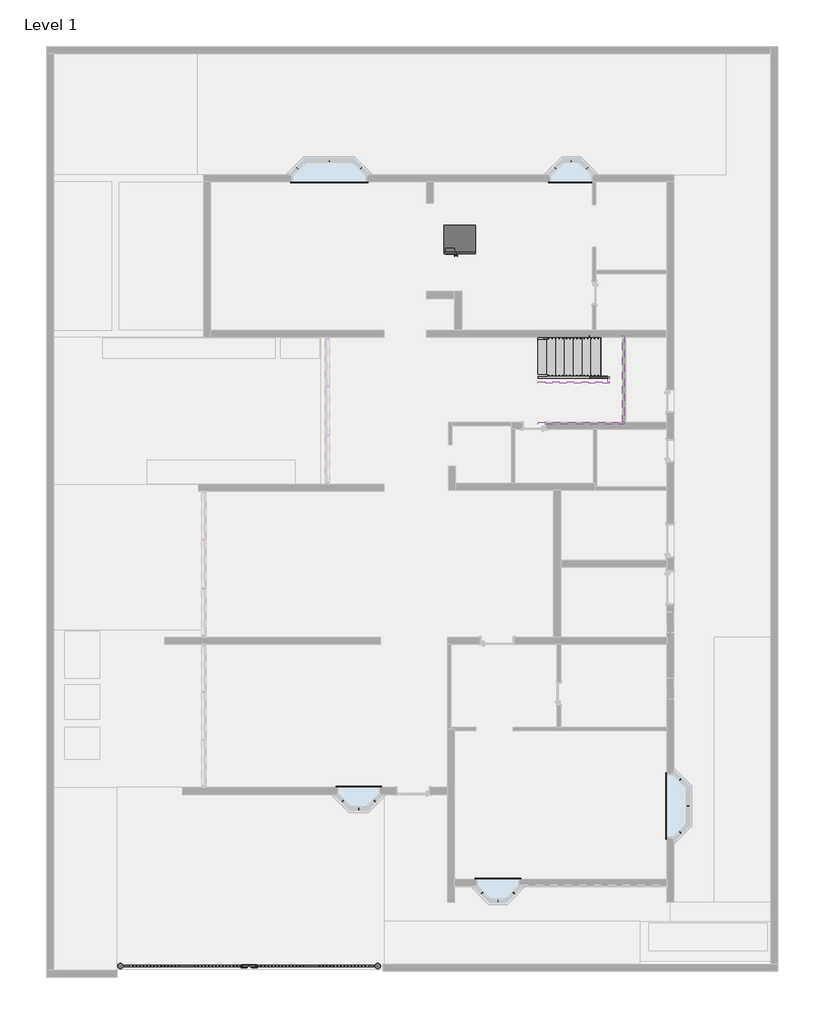
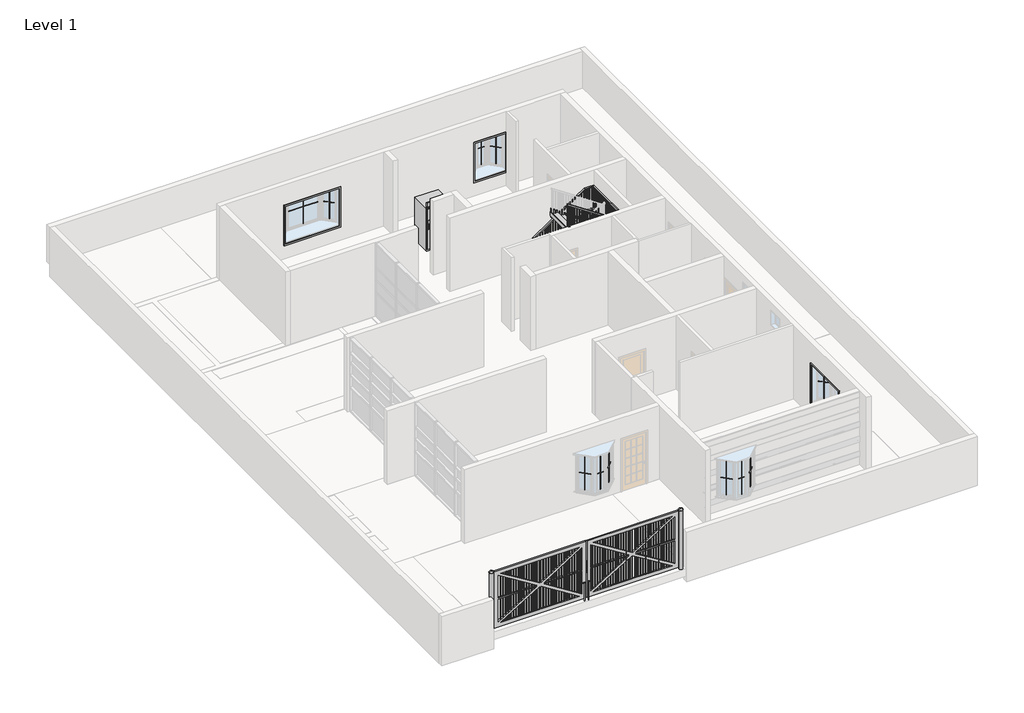
# One storey, part 5 of 5: 22 proxies, 6 members, 1 railing, 1 stair flight.
"""IFC4 building model written with IfcOpenShell, lengths in millimetres."""

from ifc_helpers import new_model, si_unit, frame, origin, place, context, project, spatial, polyline, outline, extrude, faceted_brep, transform, mapped, element, save
from components import proxy_94deb4ca, double_metal_gate_10830_double_metal_gate_10830_8bfe90f4, muntin_pattern_2x2_muntin_pattern_2x2_511ed329, muntin_pattern_2x2_muntin_pattern_2x2_63bd3b25, muntin_pattern_2x2_muntin_pattern_2x2_79566686, muntin_pattern_2x2_muntin_pattern_2x2_fa156a83, trim_window_interior_flat_picture_frame_e25f2530, trim_window_interior_flat_picture_frame_1060724f, trim_window_interior_flat_picture_frame_bf12a1e4, stair_flight_b7e44e04

model = new_model("IFC4")

# Units and contexts
model_context = context("Model", 3, world=origin())
ifc_project = project(units=[si_unit("LENGTHUNIT", "METRE", prefix="MILLI")], contexts=[model_context])

# Site, building, storey
site = spatial("IfcSite", under=ifc_project)
building = spatial("IfcBuilding", under=site)
storey = spatial("IfcBuildingStorey", under=building, Name="Level 1", Elevation=0.0)

# Proxies
placement = place(None, origin())
proxy_shape = proxy_94deb4ca(model_context)
element("IfcBuildingElementProxy", 1, Name="36\" x 70\"", ObjectType="36\" x 70\"", at=placement, inside=storey, context=model_context, shape_type="MappedRepresentation", body=[
    mapped(proxy_shape, transform((-43399.9341626, 8623.3217021, 0.0), x_axis=(1.0, 0.0, 0.0), y_axis=(0.0, 1.0, 0.0), z_axis=(0.0, 0.0, 1.0))),
])
double_metal_gate_10830_double_metal_gate_10830_shape = double_metal_gate_10830_double_metal_gate_10830_8bfe90f4(model_context)
element("IfcBuildingElementProxy", 2, Name="DOUBLE_METAL_GATE_10830 : DOUBLE_METAL_GATE_10830", ObjectType="DOUBLE_METAL_GATE_10830 : DOUBLE_METAL_GATE_10830", at=placement, inside=storey, context=model_context, shape_type="MappedRepresentation", body=[
    mapped(double_metal_gate_10830_double_metal_gate_10830_shape, transform((-48692.8486938, -12363.2913973, 0.0), x_axis=(1.0, 0.0, 0.0), y_axis=(0.0, 1.0, 0.0), z_axis=(0.0, 0.0, 1.0))),
])
muntin_pattern_2x2_muntin_pattern_2x2_shape = muntin_pattern_2x2_muntin_pattern_2x2_511ed329(model_context)
element("IfcBuildingElementProxy", 3, Name="Muntin Pattern_2x2 : Muntin Pattern_2x2", ObjectType="Muntin Pattern_2x2 : Muntin Pattern_2x2", at=placement, inside=storey, context=model_context, shape_type="MappedRepresentation", body=[
    mapped(muntin_pattern_2x2_muntin_pattern_2x2_shape, transform((-47152.5380314, 10861.8336027, 730.25), x_axis=(1.0, 0.0, 0.0), y_axis=(0.0, 1.0, 0.0), z_axis=(0.0, 0.0, 1.0))),
])
muntin_pattern_2x2_muntin_pattern_2x2_2_shape = muntin_pattern_2x2_muntin_pattern_2x2_63bd3b25(model_context)
element("IfcBuildingElementProxy", 4, Name="Muntin Pattern_2x2 : Muntin Pattern_2x2", ObjectType="Muntin Pattern_2x2 : Muntin Pattern_2x2", at=placement, inside=storey, context=model_context, shape_type="MappedRepresentation", body=[
    mapped(muntin_pattern_2x2_muntin_pattern_2x2_2_shape, transform((-48067.2297602, 10633.9378984, 730.25), x_axis=(0.7071067811865505, 0.7071067811865448, 0.0), y_axis=(-0.7071067811865448, 0.7071067811865505, 0.0), z_axis=(0.0, 0.0, 1.0))),
])
element("IfcBuildingElementProxy", 5, Name="Muntin Pattern_2x2 : Muntin Pattern_2x2", ObjectType="Muntin Pattern_2x2 : Muntin Pattern_2x2", at=placement, inside=storey, context=model_context, shape_type="MappedRepresentation", body=[
    mapped(muntin_pattern_2x2_muntin_pattern_2x2_2_shape, transform((-46237.8463026, 10633.9378984, 730.25), x_axis=(0.707106781186546, -0.7071067811865491, 0.0), y_axis=(0.7071067811865491, 0.707106781186546, 0.0), z_axis=(0.0, 0.0, 1.0))),
])
element("IfcBuildingElementProxy", 6, Name="Muntin Pattern_2x2 : Muntin Pattern_2x2", ObjectType="Muntin Pattern_2x2 : Muntin Pattern_2x2", at=placement, inside=storey, context=model_context, shape_type="MappedRepresentation", body=[
    mapped(muntin_pattern_2x2_muntin_pattern_2x2_2_shape, transform((-40650.4297602, 10633.9378984, 730.25), x_axis=(0.7071067811865505, 0.7071067811865448, 0.0), y_axis=(-0.7071067811865448, 0.7071067811865505, 0.0), z_axis=(0.0, 0.0, 1.0))),
])
element("IfcBuildingElementProxy", 7, Name="Muntin Pattern_2x2 : Muntin Pattern_2x2", ObjectType="Muntin Pattern_2x2 : Muntin Pattern_2x2", at=placement, inside=storey, context=model_context, shape_type="MappedRepresentation", body=[
    mapped(muntin_pattern_2x2_muntin_pattern_2x2_2_shape, transform((-39735.4463026, 10633.9378984, 730.25), x_axis=(0.707106781186546, -0.7071067811865491, 0.0), y_axis=(0.7071067811865491, 0.707106781186546, 0.0), z_axis=(0.0, 0.0, 1.0))),
])
element("IfcBuildingElementProxy", 8, Name="Muntin Pattern_2x2 : Muntin Pattern_2x2", ObjectType="Muntin Pattern_2x2 : Muntin Pattern_2x2", at=placement, inside=storey, context=model_context, shape_type="MappedRepresentation", body=[
    mapped(muntin_pattern_2x2_muntin_pattern_2x2_2_shape, transform((-41843.6463026, -10189.1206929, 730.25), x_axis=(-0.7071067811865505, -0.7071067811865448, 0.0), y_axis=(0.7071067811865448, -0.7071067811865505, 0.0), z_axis=(0.0, 0.0, 1.0))),
])
element("IfcBuildingElementProxy", 9, Name="Muntin Pattern_2x2 : Muntin Pattern_2x2", ObjectType="Muntin Pattern_2x2 : Muntin Pattern_2x2", at=placement, inside=storey, context=model_context, shape_type="MappedRepresentation", body=[
    mapped(muntin_pattern_2x2_muntin_pattern_2x2_2_shape, transform((-42758.6297602, -10189.1206929, 730.25), x_axis=(-0.707106781186546, 0.7071067811865491, 0.0), y_axis=(-0.7071067811865491, -0.707106781186546, 0.0), z_axis=(0.0, 0.0, 1.0))),
])
element("IfcBuildingElementProxy", 10, Name="Muntin Pattern_2x2 : Muntin Pattern_2x2", ObjectType="Muntin Pattern_2x2 : Muntin Pattern_2x2", at=placement, inside=storey, context=model_context, shape_type="MappedRepresentation", body=[
    mapped(muntin_pattern_2x2_muntin_pattern_2x2_2_shape, transform((-37058.5087357, -6927.3996684, 730.25), x_axis=(0.7071067811865458, -0.7071067811865495, 0.0), y_axis=(0.7071067811865495, 0.7071067811865458, 0.0), z_axis=(0.0, 0.0, 1.0))),
])
element("IfcBuildingElementProxy", 11, Name="Muntin Pattern_2x2 : Muntin Pattern_2x2", ObjectType="Muntin Pattern_2x2 : Muntin Pattern_2x2", at=placement, inside=storey, context=model_context, shape_type="MappedRepresentation", body=[
    mapped(muntin_pattern_2x2_muntin_pattern_2x2_2_shape, transform((-37058.5087357, -8451.9831261, 730.25), x_axis=(-0.7071067811865481, -0.707106781186547, 0.0), y_axis=(0.707106781186547, -0.7071067811865481, 0.0), z_axis=(0.0, 0.0, 1.0))),
])
element("IfcBuildingElementProxy", 12, Name="Muntin Pattern_2x2 : Muntin Pattern_2x2", ObjectType="Muntin Pattern_2x2 : Muntin Pattern_2x2", at=placement, inside=storey, context=model_context, shape_type="MappedRepresentation", body=[
    mapped(muntin_pattern_2x2_muntin_pattern_2x2_2_shape, transform((-45844.1463026, -7547.5206929, 730.25), x_axis=(-0.7071067811865506, -0.7071067811865447, 0.0), y_axis=(0.7071067811865447, -0.7071067811865506, 0.0), z_axis=(0.0, 0.0, 1.0))),
])
element("IfcBuildingElementProxy", 13, Name="Muntin Pattern_2x2 : Muntin Pattern_2x2", ObjectType="Muntin Pattern_2x2 : Muntin Pattern_2x2", at=placement, inside=storey, context=model_context, shape_type="MappedRepresentation", body=[
    mapped(muntin_pattern_2x2_muntin_pattern_2x2_2_shape, transform((-46759.1297602, -7547.5206929, 730.25), x_axis=(-0.7071067811865459, 0.7071067811865492, 0.0), y_axis=(-0.7071067811865492, -0.7071067811865459, 0.0), z_axis=(0.0, 0.0, 1.0))),
])
muntin_pattern_2x2_muntin_pattern_2x2_3_shape = muntin_pattern_2x2_muntin_pattern_2x2_79566686(model_context)
element("IfcBuildingElementProxy", 14, Name="Muntin Pattern_2x2 : Muntin Pattern_2x2", ObjectType="Muntin Pattern_2x2 : Muntin Pattern_2x2", at=placement, inside=storey, context=model_context, shape_type="MappedRepresentation", body=[
    mapped(muntin_pattern_2x2_muntin_pattern_2x2_3_shape, transform((-40192.9380314, 10861.8336027, 730.25), x_axis=(1.0, 0.0, 0.0), y_axis=(0.0, 1.0, 0.0), z_axis=(0.0, 0.0, 1.0))),
])
element("IfcBuildingElementProxy", 15, Name="Muntin Pattern_2x2 : Muntin Pattern_2x2", ObjectType="Muntin Pattern_2x2 : Muntin Pattern_2x2", at=placement, inside=storey, context=model_context, shape_type="MappedRepresentation", body=[
    mapped(muntin_pattern_2x2_muntin_pattern_2x2_3_shape, transform((-42301.1380314, -10417.0163973, 730.25), x_axis=(-1.0, 0.0, 0.0), y_axis=(0.0, -1.0, 0.0), z_axis=(0.0, 0.0, 1.0))),
])
element("IfcBuildingElementProxy", 16, Name="Muntin Pattern_2x2 : Muntin Pattern_2x2", ObjectType="Muntin Pattern_2x2 : Muntin Pattern_2x2", at=placement, inside=storey, context=model_context, shape_type="MappedRepresentation", body=[
    mapped(muntin_pattern_2x2_muntin_pattern_2x2_3_shape, transform((-46301.6380314, -7775.4163973, 730.25), x_axis=(-1.0, 0.0, 0.0), y_axis=(0.0, -1.0, 0.0), z_axis=(0.0, 0.0, 1.0))),
])
muntin_pattern_2x2_muntin_pattern_2x2_4_shape = muntin_pattern_2x2_muntin_pattern_2x2_fa156a83(model_context)
element("IfcBuildingElementProxy", 17, Name="Muntin Pattern_2x2 : Muntin Pattern_2x2", ObjectType="Muntin Pattern_2x2 : Muntin Pattern_2x2", at=placement, inside=storey, context=model_context, shape_type="MappedRepresentation", body=[
    mapped(muntin_pattern_2x2_muntin_pattern_2x2_4_shape, transform((-36830.6130314, -7689.6913973, 730.25), x_axis=(0.0, -1.0, 0.0), y_axis=(1.0, 0.0, 0.0), z_axis=(0.0, 0.0, 1.0))),
])
trim_window_interior_flat_picture_frame_shape = trim_window_interior_flat_picture_frame_e25f2530(model_context)
element("IfcBuildingElementProxy", 18, Name="Trim-Window-Interior-Flat : Picture Frame", ObjectType="Trim-Window-Interior-Flat : Picture Frame", at=placement, inside=storey, context=model_context, shape_type="MappedRepresentation", body=[
    mapped(trim_window_interior_flat_picture_frame_shape, transform((-47152.5380314, 10242.7086027, 2184.4), x_axis=(1.0, 0.0, 0.0), y_axis=(0.0, 0.0, 1.0), z_axis=(0.0, -1.0, 0.0))),
])
trim_window_interior_flat_picture_frame_2_shape = trim_window_interior_flat_picture_frame_1060724f(model_context)
element("IfcBuildingElementProxy", 19, Name="Trim-Window-Interior-Flat : Picture Frame", ObjectType="Trim-Window-Interior-Flat : Picture Frame", at=placement, inside=storey, context=model_context, shape_type="MappedRepresentation", body=[
    mapped(trim_window_interior_flat_picture_frame_2_shape, transform((-40192.9380314, 10242.7086027, 2184.4), x_axis=(1.0, 0.0, 0.0), y_axis=(0.0, 0.0, 1.0), z_axis=(0.0, -1.0, 0.0))),
])
element("IfcBuildingElementProxy", 20, Name="Trim-Window-Interior-Flat : Picture Frame", ObjectType="Trim-Window-Interior-Flat : Picture Frame", at=placement, inside=storey, context=model_context, shape_type="MappedRepresentation", body=[
    mapped(trim_window_interior_flat_picture_frame_2_shape, transform((-42301.1380314, -9797.8913973, 2184.4), x_axis=(-1.0, 0.0, 0.0), y_axis=(0.0, 0.0, 1.0), z_axis=(0.0, 1.0, 0.0))),
])
element("IfcBuildingElementProxy", 21, Name="Trim-Window-Interior-Flat : Picture Frame", ObjectType="Trim-Window-Interior-Flat : Picture Frame", at=placement, inside=storey, context=model_context, shape_type="MappedRepresentation", body=[
    mapped(trim_window_interior_flat_picture_frame_2_shape, transform((-46301.6380314, -7156.2913973, 2184.4), x_axis=(-1.0, 0.0, 0.0), y_axis=(0.0, 0.0, 1.0), z_axis=(0.0, 1.0, 0.0))),
])
trim_window_interior_flat_picture_frame_3_shape = trim_window_interior_flat_picture_frame_bf12a1e4(model_context)
element("IfcBuildingElementProxy", 22, Name="Trim-Window-Interior-Flat : Picture Frame", ObjectType="Trim-Window-Interior-Flat : Picture Frame", at=placement, inside=storey, context=model_context, shape_type="MappedRepresentation", body=[
    mapped(trim_window_interior_flat_picture_frame_3_shape, transform((-37449.7380314, -7689.6913973, 2184.4), x_axis=(0.0, -1.0, 0.0), y_axis=(0.0, 0.0, 1.0), z_axis=(-1.0, 0.0, 0.0))),
])

# Members
element("IfcMember", 23, ObjectType="Stringer - 2\" Width", at=placement, inside=storey, context=model_context, shape_type="SweptSolid", body=[
    extrude(outline(polyline([(218.0398409, -41148.2472477), (0.0, -41148.2472477), (0.0, -40925.8209948), (1470.7219756, -38719.7380314), (1600.2, -38719.7380314), (1600.2, -39075.0070091), (218.0398409, -41148.2472477)])), frame((0.0, 5772.3086027, 0.0), z_axis=(0.0, 1.0, 0.0), x_axis=(0.0, 0.0, 1.0)), (0.0, 0.0, 1.0), 50.8),
])
element("IfcMember", 24, ObjectType="Stringer - 2\" Width", at=placement, inside=storey, context=model_context, shape_type="SweptSolid", body=[
    extrude(outline(polyline([(-38719.7380314, 5823.1086027), (-38668.9380314, 5823.1086027), (-38668.9380314, 3333.9086027), (-38719.7380314, 3333.9086027), (-38719.7380314, 5823.1086027)])), frame((0.0, 0.0, 1295.4), z_axis=(0.0, 0.0, 1.0), x_axis=(1.0, 0.0, 0.0)), (0.0, 0.0, 1.0), 304.8),
])
element("IfcMember", 25, ObjectType="Stringer - 2\" Width", at=placement, inside=storey, context=model_context, shape_type="SweptSolid", body=[
    extrude(outline(polyline([(1295.4, -38668.9380314), (1443.8336967, -38668.9380314), (3096.7065076, -41148.2472477), (2730.382498, -41148.2472477), (1295.4, -38995.7735007), (1295.4, -38668.9380314)])), frame((0.0, 3283.1086027, 0.0), z_axis=(0.0, 1.0, 0.0), x_axis=(0.0, 0.0, 1.0)), (0.0, 0.0, 1.0), 50.8),
])
element("IfcMember", 26, ObjectType="Stringer - 2\" Width", at=placement, inside=storey, context=model_context, shape_type="SweptSolid", body=[
    extrude(outline(polyline([(218.0398409, -41148.2472477), (0.0, -41148.2472477), (0.0, -40925.8209948), (1189.4491647, -39141.6472477), (1555.7731743, -39141.6472477), (218.0398409, -41148.2472477)])), frame((0.0, 4603.9086027, 0.0), z_axis=(0.0, 1.0, 0.0), x_axis=(0.0, 0.0, 1.0)), (0.0, 0.0, 1.0), 50.8),
])
element("IfcMember", 27, ObjectType="Stringer - 2\" Width", at=placement, inside=storey, context=model_context, shape_type="SweptSolid", body=[
    extrude(outline(polyline([(-39141.6472477, 4654.7086027), (-39090.8472477, 4654.7086027), (-39090.8472477, 4502.3086027), (-39141.6472477, 4502.3086027), (-39141.6472477, 4654.7086027)])), frame((0.0, 0.0, 1295.4), z_axis=(0.0, 0.0, 1.0), x_axis=(1.0, 0.0, 0.0)), (0.0, 0.0, 1.0), 304.8),
])
element("IfcMember", 28, ObjectType="Stringer - 2\" Width", at=placement, inside=storey, context=model_context, shape_type="SweptSolid", body=[
    extrude(outline(polyline([(1358.782498, -39090.8472477), (1725.1065076, -39090.8472477), (3096.7065076, -41148.2472477), (2730.382498, -41148.2472477), (1358.782498, -39090.8472477)])), frame((0.0, 4451.5086027, 0.0), z_axis=(0.0, 1.0, 0.0), x_axis=(0.0, 0.0, 1.0)), (0.0, 0.0, 1.0), 50.8),
])

# Railing
element("IfcRailing", 29, ObjectType="Handrail - Rectangular", at=placement, inside=storey, context=model_context, shape_type="SolidModel", body=[
    faceted_brep([(-41148.2472477, 5772.3086027, 1083.7333333), (-41148.2472477, 5772.3086027, 1022.6793317), (-41148.2472477, 5721.5086027, 1022.6793317), (-41148.2472477, 5721.5086027, 1083.7333333), (-39116.2472477, 5772.3086027, 2438.4), (-39100.8662454, 5772.3086027, 2387.6), (-39100.8662454, 5721.5086027, 2387.6), (-39116.2472477, 5721.5086027, 2438.4), (-38719.7380314, 5772.3086027, 2438.4), (-38719.7380314, 5772.3086027, 2387.6), (-38770.5380314, 5721.5086027, 2387.6), (-38770.5380314, 5721.5086027, 2438.4), (-38719.7380314, 3333.9086027, 2438.4), (-38719.7380314, 3333.9086027, 2387.6), (-38770.5380314, 3384.7086027, 2387.6), (-38770.5380314, 3384.7086027, 2438.4), (-38862.2472477, 3333.9086027, 2438.4), (-38877.6282501, 3333.9086027, 2387.6), (-38877.6282501, 3384.7086027, 2387.6), (-38862.2472477, 3384.7086027, 2438.4), (-41148.2472477, 3333.9086027, 3962.4), (-41148.2472477, 3384.7086027, 3962.4), (-41148.2472477, 3384.7086027, 3901.3459984), (-41148.2472477, 3333.9086027, 3901.3459984)], [[[0, 1, 2, 3]], [[1, 0, 4, 5]], [[2, 1, 5, 6]], [[3, 2, 6, 7]], [[0, 3, 7, 4]], [[5, 4, 8, 9]], [[6, 5, 9, 10]], [[7, 6, 10, 11]], [[4, 7, 11, 8]], [[9, 8, 12, 13]], [[10, 9, 13, 14]], [[11, 10, 14, 15]], [[8, 11, 15, 12]], [[13, 12, 16, 17]], [[14, 13, 17, 18]], [[15, 14, 18, 19]], [[12, 15, 19, 16]], [[20, 21, 22, 23]], [[17, 16, 20, 23]], [[18, 17, 23, 22]], [[19, 18, 22, 21]], [[16, 19, 21, 20]]]),
    extrude(outline(polyline([(3863.4898542, -41091.4630314), (2878.6666667, -41091.4630314), (2878.6666667, -41072.4130314), (3850.7898542, -41072.4130314), (3863.4898542, -41091.4630314)])), frame((0.0, 3349.7836027, 0.0), z_axis=(0.0, 1.0, 0.0), x_axis=(0.0, 0.0, 1.0)), (0.0, 0.0, 1.0), 19.05),
    extrude(outline(polyline([(3795.7565208, -40989.8630314), (2878.6666667, -40989.8630314), (2878.6666667, -40970.8130314), (3783.0565208, -40970.8130314), (3795.7565208, -40989.8630314)])), frame((0.0, 3349.7836027, 0.0), z_axis=(0.0, 1.0, 0.0), x_axis=(0.0, 0.0, 1.0)), (0.0, 0.0, 1.0), 19.05),
    extrude(outline(polyline([(3728.0231875, -40888.2630314), (2709.3333333, -40888.2630314), (2709.3333333, -40869.2130314), (3715.3231875, -40869.2130314), (3728.0231875, -40888.2630314)])), frame((0.0, 3349.7836027, 0.0), z_axis=(0.0, 1.0, 0.0), x_axis=(0.0, 0.0, 1.0)), (0.0, 0.0, 1.0), 19.05),
    extrude(outline(polyline([(3660.2898542, -40786.6630314), (2709.3333333, -40786.6630314), (2709.3333333, -40767.6130314), (3647.5898542, -40767.6130314), (3660.2898542, -40786.6630314)])), frame((0.0, 3349.7836027, 0.0), z_axis=(0.0, 1.0, 0.0), x_axis=(0.0, 0.0, 1.0)), (0.0, 0.0, 1.0), 19.05),
    extrude(outline(polyline([(3592.5565208, -40685.0630314), (2709.3333333, -40685.0630314), (2709.3333333, -40666.0130314), (3579.8565208, -40666.0130314), (3592.5565208, -40685.0630314)])), frame((0.0, 3349.7836027, 0.0), z_axis=(0.0, 1.0, 0.0), x_axis=(0.0, 0.0, 1.0)), (0.0, 0.0, 1.0), 19.05),
    extrude(outline(polyline([(3524.8231875, -40583.4630314), (2540.0, -40583.4630314), (2540.0, -40564.4130314), (3512.1231875, -40564.4130314), (3524.8231875, -40583.4630314)])), frame((0.0, 3349.7836027, 0.0), z_axis=(0.0, 1.0, 0.0), x_axis=(0.0, 0.0, 1.0)), (0.0, 0.0, 1.0), 19.05),
    extrude(outline(polyline([(3457.0898542, -40481.8630314), (2540.0, -40481.8630314), (2540.0, -40462.8130314), (3444.3898542, -40462.8130314), (3457.0898542, -40481.8630314)])), frame((0.0, 3349.7836027, 0.0), z_axis=(0.0, 1.0, 0.0), x_axis=(0.0, 0.0, 1.0)), (0.0, 0.0, 1.0), 19.05),
    extrude(outline(polyline([(3389.3565208, -40380.2630314), (2370.6666667, -40380.2630314), (2370.6666667, -40361.2130314), (3376.6565208, -40361.2130314), (3389.3565208, -40380.2630314)])), frame((0.0, 3349.7836027, 0.0), z_axis=(0.0, 1.0, 0.0), x_axis=(0.0, 0.0, 1.0)), (0.0, 0.0, 1.0), 19.05),
    extrude(outline(polyline([(3321.6231875, -40278.6630314), (2370.6666667, -40278.6630314), (2370.6666667, -40259.6130314), (3308.9231875, -40259.6130314), (3321.6231875, -40278.6630314)])), frame((0.0, 3349.7836027, 0.0), z_axis=(0.0, 1.0, 0.0), x_axis=(0.0, 0.0, 1.0)), (0.0, 0.0, 1.0), 19.05),
    extrude(outline(polyline([(3253.8898542, -40177.0630314), (2370.6666667, -40177.0630314), (2370.6666667, -40158.0130314), (3241.1898542, -40158.0130314), (3253.8898542, -40177.0630314)])), frame((0.0, 3349.7836027, 0.0), z_axis=(0.0, 1.0, 0.0), x_axis=(0.0, 0.0, 1.0)), (0.0, 0.0, 1.0), 19.05),
    extrude(outline(polyline([(3186.1565208, -40075.4630314), (2201.3333333, -40075.4630314), (2201.3333333, -40056.4130314), (3173.4565208, -40056.4130314), (3186.1565208, -40075.4630314)])), frame((0.0, 3349.7836027, 0.0), z_axis=(0.0, 1.0, 0.0), x_axis=(0.0, 0.0, 1.0)), (0.0, 0.0, 1.0), 19.05),
    extrude(outline(polyline([(3118.4231875, -39973.8630314), (2201.3333333, -39973.8630314), (2201.3333333, -39954.8130314), (3105.7231875, -39954.8130314), (3118.4231875, -39973.8630314)])), frame((0.0, 3349.7836027, 0.0), z_axis=(0.0, 1.0, 0.0), x_axis=(0.0, 0.0, 1.0)), (0.0, 0.0, 1.0), 19.05),
    extrude(outline(polyline([(3050.6898542, -39872.2630314), (2032.0, -39872.2630314), (2032.0, -39853.2130314), (3037.9898542, -39853.2130314), (3050.6898542, -39872.2630314)])), frame((0.0, 3349.7836027, 0.0), z_axis=(0.0, 1.0, 0.0), x_axis=(0.0, 0.0, 1.0)), (0.0, 0.0, 1.0), 19.05),
    extrude(outline(polyline([(2982.9565208, -39770.6630314), (2032.0, -39770.6630314), (2032.0, -39751.6130314), (2970.2565208, -39751.6130314), (2982.9565208, -39770.6630314)])), frame((0.0, 3349.7836027, 0.0), z_axis=(0.0, 1.0, 0.0), x_axis=(0.0, 0.0, 1.0)), (0.0, 0.0, 1.0), 19.05),
    extrude(outline(polyline([(2915.2231875, -39669.0630314), (2032.0, -39669.0630314), (2032.0, -39650.0130314), (2902.5231875, -39650.0130314), (2915.2231875, -39669.0630314)])), frame((0.0, 3349.7836027, 0.0), z_axis=(0.0, 1.0, 0.0), x_axis=(0.0, 0.0, 1.0)), (0.0, 0.0, 1.0), 19.05),
    extrude(outline(polyline([(2847.4898542, -39567.4630314), (1862.6666667, -39567.4630314), (1862.6666667, -39548.4130314), (2834.7898542, -39548.4130314), (2847.4898542, -39567.4630314)])), frame((0.0, 3349.7836027, 0.0), z_axis=(0.0, 1.0, 0.0), x_axis=(0.0, 0.0, 1.0)), (0.0, 0.0, 1.0), 19.05),
    extrude(outline(polyline([(2779.7565208, -39465.8630314), (1862.6666667, -39465.8630314), (1862.6666667, -39446.8130314), (2767.0565208, -39446.8130314), (2779.7565208, -39465.8630314)])), frame((0.0, 3349.7836027, 0.0), z_axis=(0.0, 1.0, 0.0), x_axis=(0.0, 0.0, 1.0)), (0.0, 0.0, 1.0), 19.05),
    extrude(outline(polyline([(2712.0231875, -39364.2630314), (1693.3333333, -39364.2630314), (1693.3333333, -39345.2130314), (2699.3231875, -39345.2130314), (2712.0231875, -39364.2630314)])), frame((0.0, 3349.7836027, 0.0), z_axis=(0.0, 1.0, 0.0), x_axis=(0.0, 0.0, 1.0)), (0.0, 0.0, 1.0), 19.05),
    extrude(outline(polyline([(2644.2898542, -39262.6630314), (1693.3333333, -39262.6630314), (1693.3333333, -39243.6130314), (2631.5898542, -39243.6130314), (2644.2898542, -39262.6630314)])), frame((0.0, 3349.7836027, 0.0), z_axis=(0.0, 1.0, 0.0), x_axis=(0.0, 0.0, 1.0)), (0.0, 0.0, 1.0), 19.05),
    extrude(outline(polyline([(2576.5565208, -39161.0630314), (1693.3333333, -39161.0630314), (1693.3333333, -39142.0130314), (2563.8565208, -39142.0130314), (2576.5565208, -39161.0630314)])), frame((0.0, 3349.7836027, 0.0), z_axis=(0.0, 1.0, 0.0), x_axis=(0.0, 0.0, 1.0)), (0.0, 0.0, 1.0), 19.05),
    extrude(outline(polyline([(2508.8231875, -39059.4630314), (1524.0, -39059.4630314), (1524.0, -39040.4130314), (2496.1231875, -39040.4130314), (2508.8231875, -39059.4630314)])), frame((0.0, 3349.7836027, 0.0), z_axis=(0.0, 1.0, 0.0), x_axis=(0.0, 0.0, 1.0)), (0.0, 0.0, 1.0), 19.05),
    extrude(outline(polyline([(2441.0898542, -38957.8630314), (1524.0, -38957.8630314), (1524.0, -38938.8130314), (2428.3898542, -38938.8130314), (2441.0898542, -38957.8630314)])), frame((0.0, 3349.7836027, 0.0), z_axis=(0.0, 1.0, 0.0), x_axis=(0.0, 0.0, 1.0)), (0.0, 0.0, 1.0), 19.05),
    extrude(outline(polyline([(-38837.2130314, 3349.7836027), (-38856.2630314, 3349.7836027), (-38856.2630314, 3368.8336027), (-38837.2130314, 3368.8336027), (-38837.2130314, 3349.7836027)])), frame((0.0, 0.0, 1524.0), z_axis=(0.0, 0.0, 1.0), x_axis=(1.0, 0.0, 0.0)), (0.0, 0.0, 1.0), 863.6),
    extrude(outline(polyline([(-38735.6130314, 3419.6336027), (-38735.6130314, 3400.5836027), (-38754.6630314, 3400.5836027), (-38754.6630314, 3419.6336027), (-38735.6130314, 3419.6336027)])), frame((0.0, 0.0, 1524.0), z_axis=(0.0, 0.0, 1.0), x_axis=(1.0, 0.0, 0.0)), (0.0, 0.0, 1.0), 863.6),
    extrude(outline(polyline([(-38735.6130314, 3521.2336027), (-38735.6130314, 3502.1836027), (-38754.6630314, 3502.1836027), (-38754.6630314, 3521.2336027), (-38735.6130314, 3521.2336027)])), frame((0.0, 0.0, 1524.0), z_axis=(0.0, 0.0, 1.0), x_axis=(1.0, 0.0, 0.0)), (0.0, 0.0, 1.0), 863.6),
    extrude(outline(polyline([(-38735.6130314, 3622.8336027), (-38735.6130314, 3603.7836027), (-38754.6630314, 3603.7836027), (-38754.6630314, 3622.8336027), (-38735.6130314, 3622.8336027)])), frame((0.0, 0.0, 1524.0), z_axis=(0.0, 0.0, 1.0), x_axis=(1.0, 0.0, 0.0)), (0.0, 0.0, 1.0), 863.6),
    extrude(outline(polyline([(-38735.6130314, 3724.4336027), (-38735.6130314, 3705.3836027), (-38754.6630314, 3705.3836027), (-38754.6630314, 3724.4336027), (-38735.6130314, 3724.4336027)])), frame((0.0, 0.0, 1524.0), z_axis=(0.0, 0.0, 1.0), x_axis=(1.0, 0.0, 0.0)), (0.0, 0.0, 1.0), 863.6),
    extrude(outline(polyline([(-38735.6130314, 3826.0336027), (-38735.6130314, 3806.9836027), (-38754.6630314, 3806.9836027), (-38754.6630314, 3826.0336027), (-38735.6130314, 3826.0336027)])), frame((0.0, 0.0, 1524.0), z_axis=(0.0, 0.0, 1.0), x_axis=(1.0, 0.0, 0.0)), (0.0, 0.0, 1.0), 863.6),
    extrude(outline(polyline([(-38735.6130314, 3927.6336027), (-38735.6130314, 3908.5836027), (-38754.6630314, 3908.5836027), (-38754.6630314, 3927.6336027), (-38735.6130314, 3927.6336027)])), frame((0.0, 0.0, 1524.0), z_axis=(0.0, 0.0, 1.0), x_axis=(1.0, 0.0, 0.0)), (0.0, 0.0, 1.0), 863.6),
    extrude(outline(polyline([(-38735.6130314, 4029.2336027), (-38735.6130314, 4010.1836027), (-38754.6630314, 4010.1836027), (-38754.6630314, 4029.2336027), (-38735.6130314, 4029.2336027)])), frame((0.0, 0.0, 1524.0), z_axis=(0.0, 0.0, 1.0), x_axis=(1.0, 0.0, 0.0)), (0.0, 0.0, 1.0), 863.6),
    extrude(outline(polyline([(-38735.6130314, 4130.8336027), (-38735.6130314, 4111.7836027), (-38754.6630314, 4111.7836027), (-38754.6630314, 4130.8336027), (-38735.6130314, 4130.8336027)])), frame((0.0, 0.0, 1524.0), z_axis=(0.0, 0.0, 1.0), x_axis=(1.0, 0.0, 0.0)), (0.0, 0.0, 1.0), 863.6),
    extrude(outline(polyline([(-38735.6130314, 4232.4336027), (-38735.6130314, 4213.3836027), (-38754.6630314, 4213.3836027), (-38754.6630314, 4232.4336027), (-38735.6130314, 4232.4336027)])), frame((0.0, 0.0, 1524.0), z_axis=(0.0, 0.0, 1.0), x_axis=(1.0, 0.0, 0.0)), (0.0, 0.0, 1.0), 863.6),
    extrude(outline(polyline([(-38735.6130314, 4334.0336027), (-38735.6130314, 4314.9836027), (-38754.6630314, 4314.9836027), (-38754.6630314, 4334.0336027), (-38735.6130314, 4334.0336027)])), frame((0.0, 0.0, 1524.0), z_axis=(0.0, 0.0, 1.0), x_axis=(1.0, 0.0, 0.0)), (0.0, 0.0, 1.0), 863.6),
    extrude(outline(polyline([(-38735.6130314, 4435.6336027), (-38735.6130314, 4416.5836027), (-38754.6630314, 4416.5836027), (-38754.6630314, 4435.6336027), (-38735.6130314, 4435.6336027)])), frame((0.0, 0.0, 1524.0), z_axis=(0.0, 0.0, 1.0), x_axis=(1.0, 0.0, 0.0)), (0.0, 0.0, 1.0), 863.6),
    extrude(outline(polyline([(-38735.6130314, 4537.2336027), (-38735.6130314, 4518.1836027), (-38754.6630314, 4518.1836027), (-38754.6630314, 4537.2336027), (-38735.6130314, 4537.2336027)])), frame((0.0, 0.0, 1524.0), z_axis=(0.0, 0.0, 1.0), x_axis=(1.0, 0.0, 0.0)), (0.0, 0.0, 1.0), 863.6),
    extrude(outline(polyline([(-38735.6130314, 4638.8336027), (-38735.6130314, 4619.7836027), (-38754.6630314, 4619.7836027), (-38754.6630314, 4638.8336027), (-38735.6130314, 4638.8336027)])), frame((0.0, 0.0, 1524.0), z_axis=(0.0, 0.0, 1.0), x_axis=(1.0, 0.0, 0.0)), (0.0, 0.0, 1.0), 863.6),
    extrude(outline(polyline([(-38735.6130314, 4740.4336027), (-38735.6130314, 4721.3836027), (-38754.6630314, 4721.3836027), (-38754.6630314, 4740.4336027), (-38735.6130314, 4740.4336027)])), frame((0.0, 0.0, 1524.0), z_axis=(0.0, 0.0, 1.0), x_axis=(1.0, 0.0, 0.0)), (0.0, 0.0, 1.0), 863.6),
    extrude(outline(polyline([(-38735.6130314, 4842.0336027), (-38735.6130314, 4822.9836027), (-38754.6630314, 4822.9836027), (-38754.6630314, 4842.0336027), (-38735.6130314, 4842.0336027)])), frame((0.0, 0.0, 1524.0), z_axis=(0.0, 0.0, 1.0), x_axis=(1.0, 0.0, 0.0)), (0.0, 0.0, 1.0), 863.6),
    extrude(outline(polyline([(-38735.6130314, 4943.6336027), (-38735.6130314, 4924.5836027), (-38754.6630314, 4924.5836027), (-38754.6630314, 4943.6336027), (-38735.6130314, 4943.6336027)])), frame((0.0, 0.0, 1524.0), z_axis=(0.0, 0.0, 1.0), x_axis=(1.0, 0.0, 0.0)), (0.0, 0.0, 1.0), 863.6),
    extrude(outline(polyline([(-38735.6130314, 5045.2336027), (-38735.6130314, 5026.1836027), (-38754.6630314, 5026.1836027), (-38754.6630314, 5045.2336027), (-38735.6130314, 5045.2336027)])), frame((0.0, 0.0, 1524.0), z_axis=(0.0, 0.0, 1.0), x_axis=(1.0, 0.0, 0.0)), (0.0, 0.0, 1.0), 863.6),
    extrude(outline(polyline([(-38735.6130314, 5146.8336027), (-38735.6130314, 5127.7836027), (-38754.6630314, 5127.7836027), (-38754.6630314, 5146.8336027), (-38735.6130314, 5146.8336027)])), frame((0.0, 0.0, 1524.0), z_axis=(0.0, 0.0, 1.0), x_axis=(1.0, 0.0, 0.0)), (0.0, 0.0, 1.0), 863.6),
    extrude(outline(polyline([(-38735.6130314, 5248.4336027), (-38735.6130314, 5229.3836027), (-38754.6630314, 5229.3836027), (-38754.6630314, 5248.4336027), (-38735.6130314, 5248.4336027)])), frame((0.0, 0.0, 1524.0), z_axis=(0.0, 0.0, 1.0), x_axis=(1.0, 0.0, 0.0)), (0.0, 0.0, 1.0), 863.6),
    extrude(outline(polyline([(-38735.6130314, 5350.0336027), (-38735.6130314, 5330.9836027), (-38754.6630314, 5330.9836027), (-38754.6630314, 5350.0336027), (-38735.6130314, 5350.0336027)])), frame((0.0, 0.0, 1524.0), z_axis=(0.0, 0.0, 1.0), x_axis=(1.0, 0.0, 0.0)), (0.0, 0.0, 1.0), 863.6),
    extrude(outline(polyline([(-38735.6130314, 5451.6336027), (-38735.6130314, 5432.5836027), (-38754.6630314, 5432.5836027), (-38754.6630314, 5451.6336027), (-38735.6130314, 5451.6336027)])), frame((0.0, 0.0, 1524.0), z_axis=(0.0, 0.0, 1.0), x_axis=(1.0, 0.0, 0.0)), (0.0, 0.0, 1.0), 863.6),
    extrude(outline(polyline([(-38735.6130314, 5553.2336027), (-38735.6130314, 5534.1836027), (-38754.6630314, 5534.1836027), (-38754.6630314, 5553.2336027), (-38735.6130314, 5553.2336027)])), frame((0.0, 0.0, 1524.0), z_axis=(0.0, 0.0, 1.0), x_axis=(1.0, 0.0, 0.0)), (0.0, 0.0, 1.0), 863.6),
    extrude(outline(polyline([(-38735.6130314, 5654.8336027), (-38735.6130314, 5635.7836027), (-38754.6630314, 5635.7836027), (-38754.6630314, 5654.8336027), (-38735.6130314, 5654.8336027)])), frame((0.0, 0.0, 1524.0), z_axis=(0.0, 0.0, 1.0), x_axis=(1.0, 0.0, 0.0)), (0.0, 0.0, 1.0), 863.6),
    extrude(outline(polyline([(-38820.9722477, 5756.4336027), (-38801.9222477, 5756.4336027), (-38801.9222477, 5737.3836027), (-38820.9722477, 5737.3836027), (-38820.9722477, 5756.4336027)])), frame((0.0, 0.0, 1524.0), z_axis=(0.0, 0.0, 1.0), x_axis=(1.0, 0.0, 0.0)), (0.0, 0.0, 1.0), 863.6),
    extrude(outline(polyline([(-38922.5722477, 5756.4336027), (-38903.5222477, 5756.4336027), (-38903.5222477, 5737.3836027), (-38922.5722477, 5737.3836027), (-38922.5722477, 5756.4336027)])), frame((0.0, 0.0, 1524.0), z_axis=(0.0, 0.0, 1.0), x_axis=(1.0, 0.0, 0.0)), (0.0, 0.0, 1.0), 863.6),
    extrude(outline(polyline([(-39024.1722477, 5756.4336027), (-39005.1222477, 5756.4336027), (-39005.1222477, 5737.3836027), (-39024.1722477, 5737.3836027), (-39024.1722477, 5756.4336027)])), frame((0.0, 0.0, 1524.0), z_axis=(0.0, 0.0, 1.0), x_axis=(1.0, 0.0, 0.0)), (0.0, 0.0, 1.0), 863.6),
    extrude(outline(polyline([(2370.9959984, -39125.7722477), (1524.0, -39125.7722477), (1524.0, -39106.7222477), (2383.6959984, -39106.7222477), (2370.9959984, -39125.7722477)])), frame((0.0, 5737.3836027, 0.0), z_axis=(0.0, 1.0, 0.0), x_axis=(0.0, 0.0, 1.0)), (0.0, 0.0, 1.0), 19.05),
    extrude(outline(polyline([(2303.2626651, -39227.3722477), (1354.6666667, -39227.3722477), (1354.6666667, -39208.3222477), (2315.9626651, -39208.3222477), (2303.2626651, -39227.3722477)])), frame((0.0, 5737.3836027, 0.0), z_axis=(0.0, 1.0, 0.0), x_axis=(0.0, 0.0, 1.0)), (0.0, 0.0, 1.0), 19.05),
    extrude(outline(polyline([(2235.5293317, -39328.9722477), (1354.6666667, -39328.9722477), (1354.6666667, -39309.9222477), (2248.2293317, -39309.9222477), (2235.5293317, -39328.9722477)])), frame((0.0, 5737.3836027, 0.0), z_axis=(0.0, 1.0, 0.0), x_axis=(0.0, 0.0, 1.0)), (0.0, 0.0, 1.0), 19.05),
    extrude(outline(polyline([(2167.7959984, -39430.5722477), (1185.3333333, -39430.5722477), (1185.3333333, -39411.5222477), (2180.4959984, -39411.5222477), (2167.7959984, -39430.5722477)])), frame((0.0, 5737.3836027, 0.0), z_axis=(0.0, 1.0, 0.0), x_axis=(0.0, 0.0, 1.0)), (0.0, 0.0, 1.0), 19.05),
    extrude(outline(polyline([(2100.0626651, -39532.1722477), (1185.3333333, -39532.1722477), (1185.3333333, -39513.1222477), (2112.7626651, -39513.1222477), (2100.0626651, -39532.1722477)])), frame((0.0, 5737.3836027, 0.0), z_axis=(0.0, 1.0, 0.0), x_axis=(0.0, 0.0, 1.0)), (0.0, 0.0, 1.0), 19.05),
    extrude(outline(polyline([(2032.3293317, -39633.7722477), (1185.3333333, -39633.7722477), (1185.3333333, -39614.7222477), (2045.0293317, -39614.7222477), (2032.3293317, -39633.7722477)])), frame((0.0, 5737.3836027, 0.0), z_axis=(0.0, 1.0, 0.0), x_axis=(0.0, 0.0, 1.0)), (0.0, 0.0, 1.0), 19.05),
    extrude(outline(polyline([(1964.5959984, -39735.3722477), (1016.0, -39735.3722477), (1016.0, -39716.3222477), (1977.2959984, -39716.3222477), (1964.5959984, -39735.3722477)])), frame((0.0, 5737.3836027, 0.0), z_axis=(0.0, 1.0, 0.0), x_axis=(0.0, 0.0, 1.0)), (0.0, 0.0, 1.0), 19.05),
    extrude(outline(polyline([(1896.8626651, -39836.9722477), (1016.0, -39836.9722477), (1016.0, -39817.9222477), (1909.5626651, -39817.9222477), (1896.8626651, -39836.9722477)])), frame((0.0, 5737.3836027, 0.0), z_axis=(0.0, 1.0, 0.0), x_axis=(0.0, 0.0, 1.0)), (0.0, 0.0, 1.0), 19.05),
    extrude(outline(polyline([(1829.1293317, -39938.5722477), (846.6666667, -39938.5722477), (846.6666667, -39919.5222477), (1841.8293317, -39919.5222477), (1829.1293317, -39938.5722477)])), frame((0.0, 5737.3836027, 0.0), z_axis=(0.0, 1.0, 0.0), x_axis=(0.0, 0.0, 1.0)), (0.0, 0.0, 1.0), 19.05),
    extrude(outline(polyline([(1761.3959984, -40040.1722477), (846.6666667, -40040.1722477), (846.6666667, -40021.1222477), (1774.0959984, -40021.1222477), (1761.3959984, -40040.1722477)])), frame((0.0, 5737.3836027, 0.0), z_axis=(0.0, 1.0, 0.0), x_axis=(0.0, 0.0, 1.0)), (0.0, 0.0, 1.0), 19.05),
    extrude(outline(polyline([(1693.6626651, -40141.7722477), (846.6666667, -40141.7722477), (846.6666667, -40122.7222477), (1706.3626651, -40122.7222477), (1693.6626651, -40141.7722477)])), frame((0.0, 5737.3836027, 0.0), z_axis=(0.0, 1.0, 0.0), x_axis=(0.0, 0.0, 1.0)), (0.0, 0.0, 1.0), 19.05),
    extrude(outline(polyline([(1625.9293317, -40243.3722477), (677.3333333, -40243.3722477), (677.3333333, -40224.3222477), (1638.6293317, -40224.3222477), (1625.9293317, -40243.3722477)])), frame((0.0, 5737.3836027, 0.0), z_axis=(0.0, 1.0, 0.0), x_axis=(0.0, 0.0, 1.0)), (0.0, 0.0, 1.0), 19.05),
    extrude(outline(polyline([(1558.1959984, -40344.9722477), (677.3333333, -40344.9722477), (677.3333333, -40325.9222477), (1570.8959984, -40325.9222477), (1558.1959984, -40344.9722477)])), frame((0.0, 5737.3836027, 0.0), z_axis=(0.0, 1.0, 0.0), x_axis=(0.0, 0.0, 1.0)), (0.0, 0.0, 1.0), 19.05),
    extrude(outline(polyline([(1490.4626651, -40446.5722477), (508.0, -40446.5722477), (508.0, -40427.5222477), (1503.1626651, -40427.5222477), (1490.4626651, -40446.5722477)])), frame((0.0, 5737.3836027, 0.0), z_axis=(0.0, 1.0, 0.0), x_axis=(0.0, 0.0, 1.0)), (0.0, 0.0, 1.0), 19.05),
    extrude(outline(polyline([(1422.7293317, -40548.1722477), (508.0, -40548.1722477), (508.0, -40529.1222477), (1435.4293317, -40529.1222477), (1422.7293317, -40548.1722477)])), frame((0.0, 5737.3836027, 0.0), z_axis=(0.0, 1.0, 0.0), x_axis=(0.0, 0.0, 1.0)), (0.0, 0.0, 1.0), 19.05),
    extrude(outline(polyline([(1354.9959984, -40649.7722477), (508.0, -40649.7722477), (508.0, -40630.7222477), (1367.6959984, -40630.7222477), (1354.9959984, -40649.7722477)])), frame((0.0, 5737.3836027, 0.0), z_axis=(0.0, 1.0, 0.0), x_axis=(0.0, 0.0, 1.0)), (0.0, 0.0, 1.0), 19.05),
    extrude(outline(polyline([(1287.2626651, -40751.3722477), (338.6666667, -40751.3722477), (338.6666667, -40732.3222477), (1299.9626651, -40732.3222477), (1287.2626651, -40751.3722477)])), frame((0.0, 5737.3836027, 0.0), z_axis=(0.0, 1.0, 0.0), x_axis=(0.0, 0.0, 1.0)), (0.0, 0.0, 1.0), 19.05),
    extrude(outline(polyline([(1219.5293317, -40852.9722477), (338.6666667, -40852.9722477), (338.6666667, -40833.9222477), (1232.2293317, -40833.9222477), (1219.5293317, -40852.9722477)])), frame((0.0, 5737.3836027, 0.0), z_axis=(0.0, 1.0, 0.0), x_axis=(0.0, 0.0, 1.0)), (0.0, 0.0, 1.0), 19.05),
    extrude(outline(polyline([(1151.7959984, -40954.5722477), (169.3333333, -40954.5722477), (169.3333333, -40935.5222477), (1164.4959984, -40935.5222477), (1151.7959984, -40954.5722477)])), frame((0.0, 5737.3836027, 0.0), z_axis=(0.0, 1.0, 0.0), x_axis=(0.0, 0.0, 1.0)), (0.0, 0.0, 1.0), 19.05),
    extrude(outline(polyline([(1084.0626651, -41056.1722477), (169.3333333, -41056.1722477), (169.3333333, -41037.1222477), (1096.7626651, -41037.1222477), (1084.0626651, -41056.1722477)])), frame((0.0, 5737.3836027, 0.0), z_axis=(0.0, 1.0, 0.0), x_axis=(0.0, 0.0, 1.0)), (0.0, 0.0, 1.0), 19.05),
    extrude(outline(polyline([(-38735.6130314, 3368.8336027), (-38735.6130314, 3349.7836027), (-38754.6630314, 3349.7836027), (-38754.6630314, 3368.8336027), (-38735.6130314, 3368.8336027)])), frame((0.0, 0.0, 1524.0), z_axis=(0.0, 0.0, 1.0), x_axis=(1.0, 0.0, 0.0)), (0.0, 0.0, 1.0), 863.6),
    extrude(outline(polyline([(-38754.6630314, 5756.4336027), (-38735.6130314, 5756.4336027), (-38735.6130314, 5737.3836027), (-38754.6630314, 5737.3836027), (-38754.6630314, 5756.4336027)])), frame((0.0, 0.0, 1524.0), z_axis=(0.0, 0.0, 1.0), x_axis=(1.0, 0.0, 0.0)), (0.0, 0.0, 1.0), 863.6),
    extrude(outline(polyline([(3901.3459984, -41148.2472477), (2878.6666667, -41148.2472477), (2878.6666667, -41129.1972477), (3888.6459984, -41129.1972477), (3901.3459984, -41148.2472477)])), frame((0.0, 3349.7836027, 0.0), z_axis=(0.0, 1.0, 0.0), x_axis=(0.0, 0.0, 1.0)), (0.0, 0.0, 1.0), 19.05),
    extrude(outline(polyline([(1022.6793317, -41148.2472477), (169.3333333, -41148.2472477), (169.3333333, -41129.1972477), (1035.3793317, -41129.1972477), (1022.6793317, -41148.2472477)])), frame((0.0, 5737.3836027, 0.0), z_axis=(0.0, 1.0, 0.0), x_axis=(0.0, 0.0, 1.0)), (0.0, 0.0, 1.0), 19.05),
])

# Stair flight
stair_flight_shape = stair_flight_b7e44e04(model_context)
element("IfcStairFlight", 30, ObjectType="2\" Tread 1\" Nosing 1/4\" Riser", at=placement, inside=storey, context=model_context, shape_type="MappedRepresentation", body=[
    mapped(stair_flight_shape, transform((0.0, 0.0, 0.0), x_axis=(1.0, 0.0, 0.0), y_axis=(0.0, 1.0, 0.0), z_axis=(0.0, 0.0, 1.0))),
])

save(model, "model.ifc")

# Revit data of these elements
# Type "36\" x 70\""
#   URL = "\r\n"
#   Label = "REF."
#   Unit_Width = 2' - 11 3/4"
#   Unit_Height = 5' - 9 1/2"
#   Unit_Depth = 2' - 8 1/2"
#   Cover_Height = 0' - 10"
#   Rigth_Door_width = 1' - 10"
#   Door_Height = 5' - 5"
#   Bottom_of_dispenser = 3' - 0"
#   Base_Height = 0' - 3 1/2"
#   Material = Metal - Stainless Steel
#   Default Elevation = 0
#   Model = ""
#   Manufacturer = ""
#   Description = (empty or 0)
#   Assembly Code = ""
# Type "DOUBLE_METAL_GATE_10830 : DOUBLE_METAL_GATE_10830"
#   WIDTH [instance default] = 24' - 0"
#   Default Elevation = 0
#   Assembly Code = ""
# Type "Muntin Pattern_2x2 : Muntin Pattern_2x2"
#   Width [instance default] = 4' - 0"
#   Thickness = 0' - 0 1/2"
#   Height [instance default] = 4' - 0"
#   Distance = 0' - 0 3/4"
#   Interior Material [instance default] = none
#   Exterior Material [instance default] = none
#   Default Elevation = 0
# Type "Trim-Window-Interior-Flat : Picture Frame"
#   Trim Thickness_Picture Frame = 0' - 1 1/4"
#   Trim Width = 0' - 2 1/4"
#   Trim Thickness_with Sill = 0' - 0 3/4"
#   Sill Thickness = 0' - 1 1/4"
#   Opening Width [instance default] = 2' - 0"
#   Opening Height [instance default] = 3' - 0"
#   Default Elevation = 4' - 0"
#   Sill = no
#   Picture Frame = yes
#   Trim Material [instance default] = none
# Type "Handrail - Rectangular"
#   Assembly Code = "C2010400"
#   built-in parameter 1008612 = 0.0416667 (stored number, unit not read)
#   built-in parameter 1008611 = 0.0416667 (stored number, unit not read)
#   built-in parameter 1008609 = 0.333333 (stored number, unit not read)
#   built-in parameter 1008604 = 0.166667 (stored number, unit not read)
#   built-in parameter 1008603 = 0.166667 (stored number, unit not read)
#   Railing Height = 3' - 0"
#   built-in parameter 1008630 = 2
#   built-in parameter 1008610 = 2
#   built-in parameter 1008618 = Baluster - Square : 3/4"
# Element 1 (IfcBuildingElementProxy, "36\" x 70\"")
#   Phase Created = New Construction
#   Materials on its faces: "Metal - Stainless Steel", "High Gloss Black"
# Element 2 (IfcBuildingElementProxy, "DOUBLE_METAL_GATE_10830 : DOUBLE_METAL_GATE_10830")
#   WIDTH = 23' - 9.2843"
#   Phase Created = New Construction
#   Materials on its faces: "Default"
# Element 3 (IfcBuildingElementProxy, "Muntin Pattern_2x2 : Muntin Pattern_2x2")
#   Width = 3' - 8.88909"
#   Height = 4' - 6 1/2"
#   Interior Material = Wood - Stained
#   Exterior Material = Clad - White
#   Phase Created = New Construction
#   Materials on its faces: "Clad - White", "Wood - Stained"
# Elements 4, 5, 6, 7, 8, 9, 10, 11, 12, 13 (IfcBuildingElementProxy, "Muntin Pattern_2x2 : Muntin Pattern_2x2")
#   Width = 1' - 4.18808"
#   Height = 4' - 6 1/2"
#   Interior Material = Wood - Stained
#   Exterior Material = Clad - White
#   Phase Created = New Construction
#   Materials on its faces: "Clad - White", "Wood - Stained"
# Elements 14, 15, 16 (IfcBuildingElementProxy, "Muntin Pattern_2x2 : Muntin Pattern_2x2")
#   Width = 0' - 8.88909"
#   Height = 4' - 6 1/2"
#   Interior Material = Wood - Stained
#   Exterior Material = Clad - White
#   Phase Created = New Construction
#   Materials on its faces: "Clad - White", "Wood - Stained"
# Element 17 (IfcBuildingElementProxy, "Muntin Pattern_2x2 : Muntin Pattern_2x2")
#   Width = 2' - 8.88909"
#   Height = 4' - 6 1/2"
#   Interior Material = Wood - Stained
#   Exterior Material = Clad - White
#   Phase Created = New Construction
#   Materials on its faces: "Clad - White", "Wood - Stained"
# Element 18 (IfcBuildingElementProxy, "Trim-Window-Interior-Flat : Picture Frame")
#   Opening Width = 7' - 0"
#   Opening Height = 5' - 2"
#   Trim Material = Wood - Stained
#   Phase Created = New Construction
#   Materials on its faces: "Wood - Stained"
# Elements 19, 20, 21 (IfcBuildingElementProxy, "Trim-Window-Interior-Flat : Picture Frame")
#   Opening Width = 4' - 0"
#   Opening Height = 5' - 2"
#   Trim Material = Wood - Stained
#   Phase Created = New Construction
#   Materials on its faces: "Wood - Stained"
# Element 22 (IfcBuildingElementProxy, "Trim-Window-Interior-Flat : Picture Frame")
#   Opening Width = 6' - 0"
#   Opening Height = 5' - 2"
#   Trim Material = Wood - Stained
#   Phase Created = New Construction
#   Materials on its faces: "Wood - Stained"
# Elements 23, 24, 25, 26, 27, 28 (IfcMember, "Stringer - 2\" Width")
#   Phase Created = New Construction
# Element 29 (IfcRailing, "Handrail - Rectangular")
#   Phase Created = New Construction
# Element 30 (IfcStairFlight, "2\" Tread 1\" Nosing 1/4\" Riser")
#   Phase Created = New Construction
# Materials
#   "Metal - Stainless Steel": colour RGB 189 187 185, transparency 0
#   "High Gloss Black": class "Metal", colour RGB 70 70 70, transparency 0
#   "Default": colour RGB 127 127 127, transparency 0, Cost = 0
#   "Clad - White": class "Wood", colour RGB 242 242 238, transparency 0, Cost = 0
#   "Wood - Stained": class "Wood", colour RGB 224 178 126, transparency 0, Cost = 0
